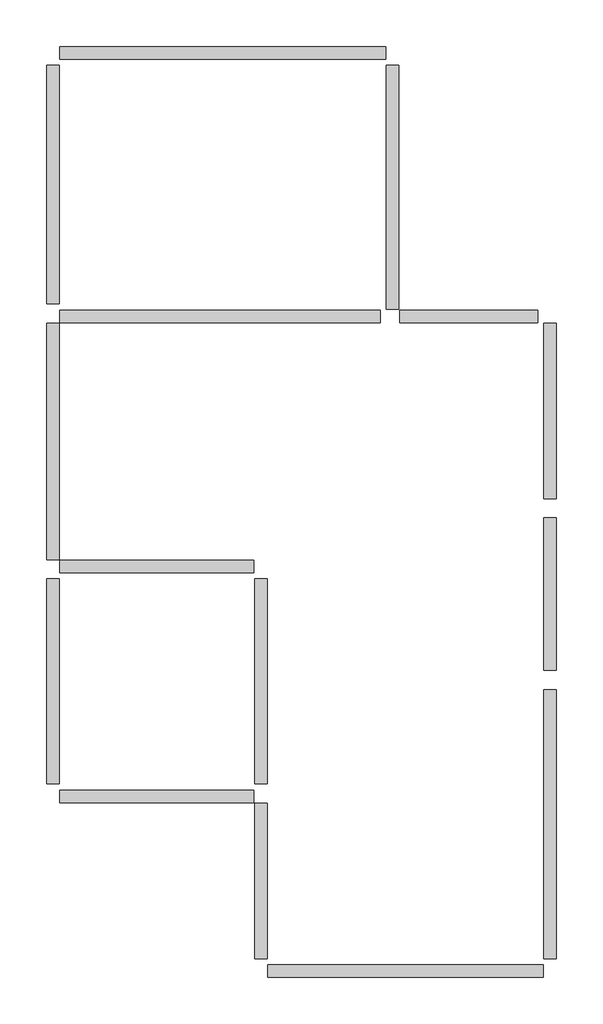
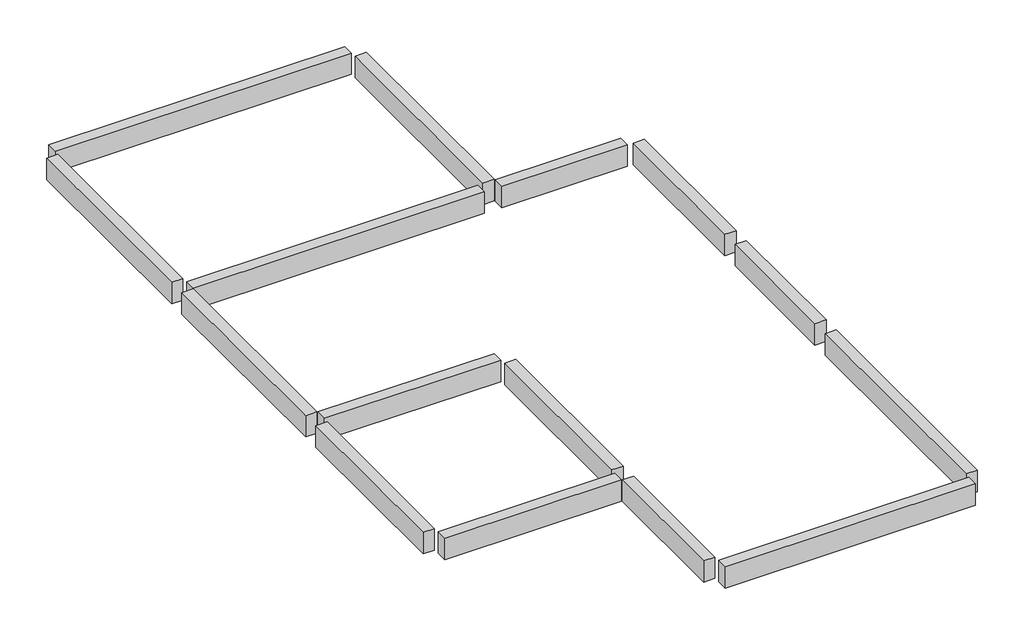
# One storey: 15 beams.
"""IFC4 building model written with IfcOpenShell, lengths in millimetres."""

from ifc_helpers import new_model, si_unit, frame, origin, place, context, project, spatial, polyline, outline, extrude, element, save

model = new_model("IFC4")

# Units and contexts
model_context = context("Model", 3, world=origin())
ifc_project = project(units=[si_unit("LENGTHUNIT", "METRE", prefix="MILLI")], contexts=[model_context])

# Site, building, storey
site = spatial("IfcSite", under=ifc_project)
building = spatial("IfcBuilding", under=site)
storey = spatial("IfcBuildingStorey", under=building, Elevation=6400.8)

# Beams
placement = place(None, origin())
element("IfcBeam", 1, ObjectType="Concrete-Rectangular Beam : 10\" x 24\"", at=placement, inside=storey, context=model_context, shape_type="SweptSolid", body=[
    extrude(outline(polyline([(-12235.0833659, 12888.2783402), (-12235.0833659, 13116.8783402), (-6266.0833659, 13116.8783402), (-6266.0833659, 12888.2783402), (-12235.0833659, 12888.2783402)])), frame((0.0, 0.0, 5943.6), z_axis=(0.0, 0.0, 1.0), x_axis=(1.0, 0.0, 0.0)), (0.0, 0.0, 1.0), 457.2),
])
element("IfcBeam", 2, ObjectType="Concrete-Rectangular Beam : 10\" x 24\"", at=placement, inside=storey, context=model_context, shape_type="SweptSolid", body=[
    extrude(outline(polyline([(-6253.3833659, 12773.9783402), (-6024.7833659, 12773.9783402), (-6024.7833659, 8303.5783402), (-6253.3833659, 8303.5783402), (-6253.3833659, 12773.9783402)])), frame((0.0, 0.0, 5943.6), z_axis=(0.0, 0.0, 1.0), x_axis=(1.0, 0.0, 0.0)), (0.0, 0.0, 1.0), 457.2),
])
element("IfcBeam", 3, ObjectType="Concrete-Rectangular Beam : 10\" x 24\"", at=placement, inside=storey, context=model_context, shape_type="SweptSolid", body=[
    extrude(outline(polyline([(-3484.7833659, 8290.8783402), (-3484.7833659, 8062.2783402), (-6012.0833659, 8062.2783402), (-6012.0833659, 8290.8783402), (-3484.7833659, 8290.8783402)])), frame((0.0, 0.0, 5943.6), z_axis=(0.0, 0.0, 1.0), x_axis=(1.0, 0.0, 0.0)), (0.0, 0.0, 1.0), 457.2),
])
element("IfcBeam", 4, ObjectType="Concrete-Rectangular Beam : 10\" x 24\"", at=placement, inside=storey, context=model_context, shape_type="SweptSolid", body=[
    extrude(outline(polyline([(-3142.0191189, 4841.8494441), (-3370.6191189, 4841.8494441), (-3370.6191189, 8049.5783402), (-3142.0191189, 8049.5783402), (-3142.0191189, 4841.8494441)])), frame((0.0, 0.0, 5943.6), z_axis=(0.0, 0.0, 1.0), x_axis=(1.0, 0.0, 0.0)), (0.0, 0.0, 1.0), 457.2),
])
element("IfcBeam", 5, ObjectType="Concrete-Rectangular Beam : 10\" x 24\"", at=placement, inside=storey, context=model_context, shape_type="SweptSolid", body=[
    extrude(outline(polyline([(-3142.0191189, 1700.3598175), (-3370.6191189, 1700.3598175), (-3370.6191189, 4486.2494441), (-3142.0191189, 4486.2494441), (-3142.0191189, 1700.3598175)])), frame((0.0, 0.0, 5943.6), z_axis=(0.0, 0.0, 1.0), x_axis=(1.0, 0.0, 0.0)), (0.0, 0.0, 1.0), 457.2),
])
element("IfcBeam", 6, ObjectType="Concrete-Rectangular Beam : 10\" x 24\"", at=placement, inside=storey, context=model_context, shape_type="SweptSolid", body=[
    extrude(outline(polyline([(-3370.6191189, 1344.7598175), (-3142.0191189, 1344.7598175), (-3142.0191189, -3583.6216598), (-3370.6191189, -3583.6216598), (-3370.6191189, 1344.7598175)])), frame((0.0, 0.0, 5943.6), z_axis=(0.0, 0.0, 1.0), x_axis=(1.0, 0.0, 0.0)), (0.0, 0.0, 1.0), 457.2),
])
element("IfcBeam", 7, ObjectType="Concrete-Rectangular Beam : 10\" x 24\"", at=placement, inside=storey, context=model_context, shape_type="SweptSolid", body=[
    extrude(outline(polyline([(-3383.3191189, -3697.9216598), (-3383.3191189, -3926.5216598), (-8425.0833659, -3926.5216598), (-8425.0833659, -3697.9216598), (-3383.3191189, -3697.9216598)])), frame((0.0, 0.0, 5943.6), z_axis=(0.0, 0.0, 1.0), x_axis=(1.0, 0.0, 0.0)), (0.0, 0.0, 1.0), 457.2),
])
element("IfcBeam", 8, ObjectType="Concrete-Rectangular Beam : 10\" x 24\"", at=placement, inside=storey, context=model_context, shape_type="SweptSolid", body=[
    extrude(outline(polyline([(-8437.7833659, -3583.6216598), (-8666.3833659, -3583.6216598), (-8666.3833659, -738.8216598), (-8437.7833659, -738.8216598), (-8437.7833659, -3583.6216598)])), frame((0.0, 0.0, 5943.6), z_axis=(0.0, 0.0, 1.0), x_axis=(1.0, 0.0, 0.0)), (0.0, 0.0, 1.0), 457.2),
])
element("IfcBeam", 9, ObjectType="Concrete-Rectangular Beam : 10\" x 24\"", at=placement, inside=storey, context=model_context, shape_type="SweptSolid", body=[
    extrude(outline(polyline([(-8666.3833659, 3369.6283402), (-8437.7833659, 3369.6283402), (-8437.7833659, -383.2216598), (-8666.3833659, -383.2216598), (-8666.3833659, 3369.6283402)])), frame((0.0, 0.0, 5943.6), z_axis=(0.0, 0.0, 1.0), x_axis=(1.0, 0.0, 0.0)), (0.0, 0.0, 1.0), 457.2),
])
element("IfcBeam", 10, ObjectType="Concrete-Rectangular Beam : 10\" x 24\"", at=placement, inside=storey, context=model_context, shape_type="SweptSolid", body=[
    extrude(outline(polyline([(-12235.0833659, 3483.9283402), (-12235.0833659, 3712.5283402), (-8679.0833659, 3712.5283402), (-8679.0833659, 3483.9283402), (-12235.0833659, 3483.9283402)])), frame((0.0, 0.0, 5943.6), z_axis=(0.0, 0.0, 1.0), x_axis=(1.0, 0.0, 0.0)), (0.0, 0.0, 1.0), 457.2),
])
element("IfcBeam", 11, ObjectType="Concrete-Rectangular Beam : 10\" x 24\"", at=placement, inside=storey, context=model_context, shape_type="SweptSolid", body=[
    extrude(outline(polyline([(-12247.7833659, -383.2216598), (-12476.3833659, -383.2216598), (-12476.3833659, 3369.6283402), (-12247.7833659, 3369.6283402), (-12247.7833659, -383.2216598)])), frame((0.0, 0.0, 5943.6), z_axis=(0.0, 0.0, 1.0), x_axis=(1.0, 0.0, 0.0)), (0.0, 0.0, 1.0), 457.2),
])
element("IfcBeam", 12, ObjectType="Concrete-Rectangular Beam : 10\" x 24\"", at=placement, inside=storey, context=model_context, shape_type="SweptSolid", body=[
    extrude(outline(polyline([(-12235.0833659, -726.1216598), (-12235.0833659, -497.5216598), (-8679.0833659, -497.5216598), (-8679.0833659, -726.1216598), (-12235.0833659, -726.1216598)])), frame((0.0, 0.0, 5943.6), z_axis=(0.0, 0.0, 1.0), x_axis=(1.0, 0.0, 0.0)), (0.0, 0.0, 1.0), 457.2),
])
element("IfcBeam", 13, ObjectType="Concrete-Rectangular Beam : 10\" x 24\"", at=placement, inside=storey, context=model_context, shape_type="SweptSolid", body=[
    extrude(outline(polyline([(-12247.7833659, 3725.2283402), (-12476.3833659, 3725.2283402), (-12476.3833659, 8049.5783402), (-12247.7833659, 8049.5783402), (-12247.7833659, 3725.2283402)])), frame((0.0, 0.0, 5943.6), z_axis=(0.0, 0.0, 1.0), x_axis=(1.0, 0.0, 0.0)), (0.0, 0.0, 1.0), 457.2),
])
element("IfcBeam", 14, ObjectType="Concrete-Rectangular Beam : 10\" x 24\"", at=placement, inside=storey, context=model_context, shape_type="SweptSolid", body=[
    extrude(outline(polyline([(-12247.7833659, 8405.1783402), (-12476.3833659, 8405.1783402), (-12476.3833659, 12773.9783402), (-12247.7833659, 12773.9783402), (-12247.7833659, 8405.1783402)])), frame((0.0, 0.0, 5943.6), z_axis=(0.0, 0.0, 1.0), x_axis=(1.0, 0.0, 0.0)), (0.0, 0.0, 1.0), 457.2),
])
element("IfcBeam", 15, ObjectType="Concrete-Rectangular Beam : 10\" x 24\"", at=placement, inside=storey, context=model_context, shape_type="SweptSolid", body=[
    extrude(outline(polyline([(-6367.6833659, 8290.8783402), (-6367.6833659, 8062.2783402), (-12235.0833659, 8062.2783402), (-12235.0833659, 8290.8783402), (-6367.6833659, 8290.8783402)])), frame((0.0, 0.0, 5943.6), z_axis=(0.0, 0.0, 1.0), x_axis=(1.0, 0.0, 0.0)), (0.0, 0.0, 1.0), 457.2),
])

save(model, "model.ifc")

# Revit data of these elements
# Type "Concrete-Rectangular Beam : 10\" x 24\""
#   Assembly Code = "B10"
#   Length [instance default] = 5' - 0"
#   b = 0' - 9"
#   h = 1' - 6"
#   Structural Material [instance default] = Concrete, Cast-in-Place gray
# Elements 1, 2, 3, 4, 5, 6, 7, 8, 9, 10, 11, 12, 13, 14, 15 (IfcBeam, "Concrete-Rectangular Beam : 10\" x 24\"")
#   Structural Material = Concrete, Cast-in-Place gray
#   Phase Created = New Construction
#   Materials on its faces: "Concrete, Cast-in-Place gray"
# Materials
#   "Concrete, Cast-in-Place gray": class "Concrete", colour RGB 192 192 192, transparency 0, Description = "Cast-in-place concrete", Cost = 0
